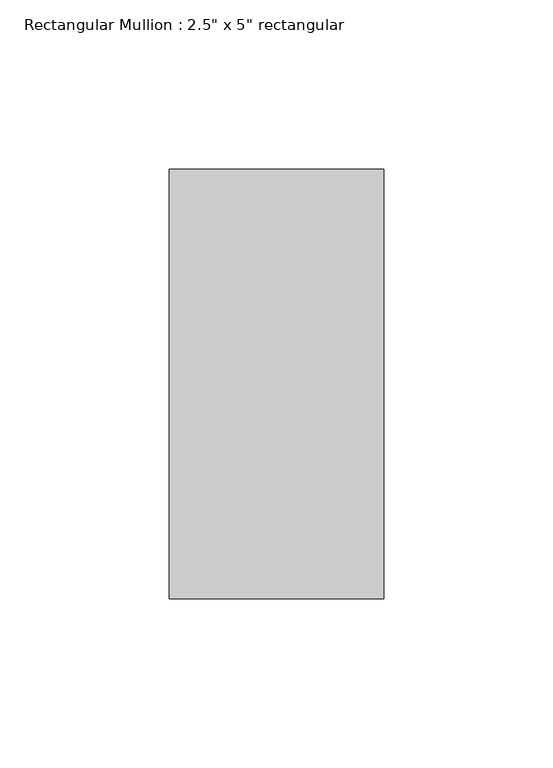
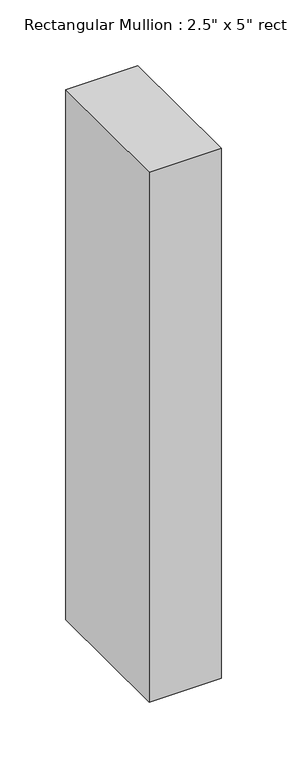
"""IFC4 building model written with IfcOpenShell, lengths in millimetres: member geometry."""

from ifc_helpers import new_model, si_unit, frame, origin, place, context, project, spatial, polyline, outline, extrude, source, transform, mapped, element, save


def member_19e7b172(model_context):
    return source(origin(), model_context, "Body", "SweptSolid", [
        extrude(outline(polyline([(0.0, 63.5), (0.0, -63.5), (-63.5, -63.5), (-63.5, 63.5), (0.0, 63.5)])), frame((0.0, 0.0, -492.8323651), z_axis=(0.0, 0.0, 1.0), x_axis=(1.0, 0.0, 0.0)), (0.0, 0.0, 1.0), 492.8323651),
    ])


if __name__ == "__main__":
    model = new_model("IFC4")
    model_context = context("Model", 3, world=origin())
    ifc_project = project(units=[si_unit("LENGTHUNIT", "METRE", prefix="MILLI")], contexts=[model_context])
    site = spatial("IfcSite", under=ifc_project)
    building = spatial("IfcBuilding", under=site)
    placement = place(None, origin())
    member_shape = member_19e7b172(model_context)
    element("IfcMember", 1, ObjectType="Rectangular Mullion : 2.5\" x 5\" rectangular", at=placement, inside=building, context=model_context, shape_type="MappedRepresentation", body=[
        mapped(member_shape, transform((0.0, 0.0, 0.0), x_axis=(1.0, 0.0, 0.0), y_axis=(0.0, 1.0, 0.0), z_axis=(0.0, 0.0, 1.0))),
    ])
    save(model, "model.ifc")

# Revit data of these elements
# Type "Rectangular Mullion : 2.5\" x 5\" rectangular"
#   built-in parameter 1007304 = 0.416667 (stored number, unit not read)
#   built-in parameter 1007301 = 0.104167 (stored number, unit not read)
#   built-in parameter 1007300 = 0.104167 (stored number, unit not read)
# Element 1 (IfcMember, "Rectangular Mullion : 2.5\" x 5\" rectangular")
#   Materials on its faces: "Aluminum"
# Materials
#   "Aluminum": class "Metal", colour RGB 247 247 247, transparency 0, Description = "Aluminum 6061", Cost = 0
